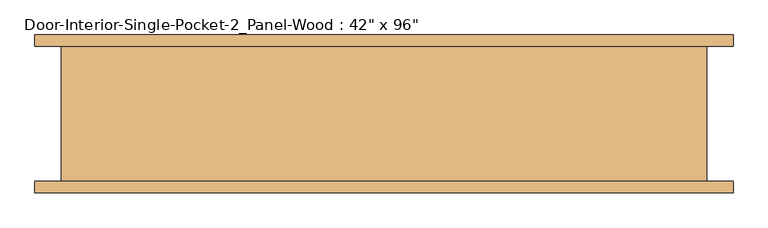
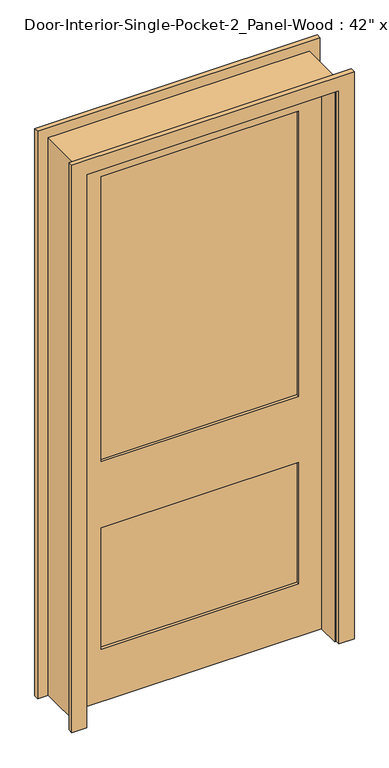
"""IFC4 building model written with IfcOpenShell, lengths in millimetres: door geometry."""

from ifc_helpers import new_model, si_unit, frame, origin, place, context, project, spatial, polyline, outline, extrude, faceted_brep, source, transform, mapped, element, save


def door_07f5c701(model_context):
    return source(origin(), model_context, "Body", "SolidModel", [
        extrude(outline(polyline([(0.0, 514.35), (0.0, 577.85), (2508.25, 577.85), (2508.25, -603.25), (0.0, -603.25), (0.0, -539.75), (2444.75, -539.75), (2444.75, 514.35), (0.0, 514.35)])), frame((0.0, 114.3, 0.0), z_axis=(0.0, 1.0, 0.0), x_axis=(0.0, 0.0, 1.0)), (0.0, 0.0, 1.0), 19.05),
        extrude(outline(polyline([(0.0, 514.35), (0.0, 577.85), (2508.25, 577.85), (2508.25, -603.25), (0.0, -603.25), (0.0, -539.75), (2444.75, -539.75), (2444.75, 514.35), (0.0, 514.35)])), frame((0.0, -133.35, 0.0), z_axis=(0.0, 1.0, 0.0), x_axis=(0.0, 0.0, 1.0)), (0.0, 0.0, 1.0), 19.05),
        extrude(outline(polyline([(2438.4, -533.4), (0.0, -533.4), (0.0, 533.4), (2438.4, 533.4), (2438.4, -533.4)]), holes=[polyline([(2319.3375, -412.75), (2319.3375, 412.75), (1060.45, 412.75), (1060.45, -412.75), (2319.3375, -412.75)]), polyline([(768.35, -412.75), (768.35, 412.75), (231.775, 412.75), (231.775, -412.75), (768.35, -412.75)])]), frame((0.0, -17.4625, 0.0), z_axis=(0.0, 1.0, 0.0), x_axis=(0.0, 0.0, 1.0)), (0.0, 0.0, 1.0), 34.925),
        extrude(outline(polyline([(412.75, -5.8208333), (-412.75, -5.8208333), (-412.75, 5.8208333), (412.75, 5.8208333), (412.75, -5.8208333)])), frame((0.0, 0.0, 1060.45), z_axis=(0.0, 0.0, 1.0), x_axis=(1.0, 0.0, 0.0)), (0.0, 0.0, 1.0), 1258.8875),
        extrude(outline(polyline([(412.75, -5.8208333), (-412.75, -5.8208333), (-412.75, 5.8208333), (412.75, 5.8208333), (412.75, -5.8208333)])), frame((0.0, 0.0, 231.775), z_axis=(0.0, 0.0, 1.0), x_axis=(1.0, 0.0, 0.0)), (0.0, 0.0, 1.0), 536.575),
        faceted_brep([(533.4, -114.3, 0.0), (533.4, -17.4625, 0.0), (533.4, -17.4625, 2438.4), (533.4, 17.4625, 2438.4), (533.4, 17.4625, 0.0), (533.4, 114.3, 0.0), (533.4, 114.3, 2463.8), (533.4, -114.3, 2463.8), (-558.8, -114.3, 2463.8), (-558.8, -114.3, 0.0), (-533.4, -114.3, 0.0), (-533.4, -114.3, 2438.4), (508.0, -114.3, 2438.4), (508.0, -114.3, 0.0), (-533.4, 114.3, 2438.4), (508.0, 114.3, 2438.4), (508.0, 17.4625, 2438.4), (508.0, -17.4625, 2438.4), (508.0, 114.3, 0.0), (-533.4, 114.3, 0.0), (-558.8, 114.3, 0.0), (-558.8, 114.3, 2463.8), (508.0, -17.4625, 0.0), (508.0, 17.4625, 0.0)], [[[0, 1, 2, 3, 4, 5, 6, 7]], [[0, 7, 8, 9, 10, 11, 12, 13]], [[11, 14, 15, 16, 3, 2, 17, 12]], [[6, 5, 18, 15, 14, 19, 20, 21]], [[6, 21, 8, 7]], [[10, 9, 20, 19]], [[11, 10, 19, 14]], [[9, 8, 21, 20]], [[1, 0, 13, 22]], [[5, 4, 23, 18]], [[18, 23, 16, 15]], [[23, 4, 3, 16]], [[1, 22, 17, 2]], [[22, 13, 12, 17]]]),
    ])


if __name__ == "__main__":
    model = new_model("IFC4")
    model_context = context("Model", 3, world=origin())
    ifc_project = project(units=[si_unit("LENGTHUNIT", "METRE", prefix="MILLI")], contexts=[model_context])
    site = spatial("IfcSite", under=ifc_project)
    building = spatial("IfcBuilding", under=site)
    placement = place(None, origin())
    door_shape = door_07f5c701(model_context)
    element("IfcDoor", 1, ObjectType="Door-Interior-Single-Pocket-2_Panel-Wood : 42\" x 96\"", at=placement, inside=building, context=model_context, shape_type="MappedRepresentation", body=[
        mapped(door_shape, transform((0.0, 0.0, 0.0), x_axis=(1.0, 0.0, 0.0), y_axis=(0.0, 1.0, 0.0), z_axis=(0.0, 0.0, 1.0))),
    ])
    save(model, "model.ifc")

# Revit data of these elements
# Type "Door-Interior-Single-Pocket-2_Panel-Wood : 42\" x 96\""
#   Type Mark = "12"
#   Assembly Code = "C1020300"
#   Analytic Construction = "Wooden"
#   Top Rail = 0' - 4 11/16"
#   Thickness = 0' - 1 3/8"
#   Thermal Resistance (R) = 2.5876 (h·ft²·°F)/BTU
#   Stiles = 0' - 4 3/4"
#   Rough Width = 7' - 1"
#   Rough Height = 8' - 4 1/2"
#   Lock Rail = 0' - 7 1/2"
#   Location [instance default] = 3' - 6"
#   Height = 8' - 0"
#   Width = 3' - 6"
#   Heat Transfer Coefficient (U) = 0.3865 BTU/(h·ft²·°F)
#   Bottom Rail = 0' - 9 1/8"
#   Panel Open [instance default] = no
#   Trim Material = Cherry
#   Panel Material = Cherry
#   Frame Material = Cherry
#   Visual Light Transmittance = 0
#   Solar Heat Gain Coefficient = 0
#   Wall Closure = (empty or 0)
#   Function = (empty or 0)
# Element 1 (IfcDoor, "Door-Interior-Single-Pocket-2_Panel-Wood : 42\" x 96\"")
#   Materials on its faces: "Cherry"
# Materials
#   "Cherry": class "Wood", colour RGB 226 177 128, transparency 0, Description = "Prunus Serotina", Cost = 0
